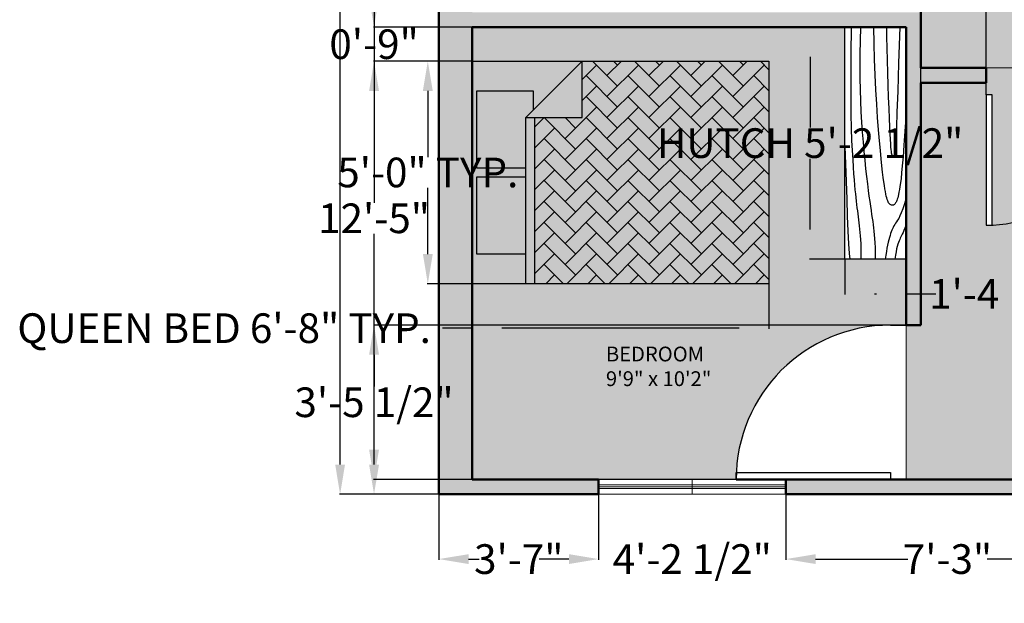
# Model space of a CAD drawing. Units: inches. Extents: x 339 to 824, y 73 to 445.
# Tile 1 of 5: x 339 to 605, y 73 to 230. Entities that reach past the tile are written whole.
import ezdxf

# ---------------------------------------------------------------- set-up
doc = ezdxf.new("R2010")
doc.units = ezdxf.units.IN
doc.header["$MEASUREMENT"] = 0
for name, color, linetype, lineweight in [('A-ANNO-DIMS', 2, 'Continuous', 18), ('A-AREA-IDEN', 7, 'Continuous', 25), ('A-DOOR', 3, 'Continuous', 25), ('A-FLOR-BNDY', 8, 'Continuous', 13), ('A-FLOR-PATT', 8, 'Continuous', 13), ('A-FURN', 9, 'Continuous', 25), ('A-FURN-FABR-PATT', 7, 'Continuous', 13), ('A-GLAZ', 4, 'Continuous', 18), ('A-WALL', 7, 'Continuous', 50), ('A-WALL-PATT', 1, 'Continuous', 13)]:
    doc.layers.add(name, color=color, linetype=linetype, lineweight=lineweight)
doc.layers.add('A-FURN-PATT', color=251, linetype='Continuous', lineweight=13, true_color=0x6d5f6c)
doc.styles.get("Standard").update_dxf_attribs({"font": 'arial.ttf'})
doc.dimstyles.get("Standard").update_dxf_attribs({"dimtxt": 8, "dimasz": 8, "dimexe": 0.18, "dimexo": 0.0625, "dimgap": 0.09, "dimtad": 0, "dimtih": 1, "dimtoh": 1, "dimdec": 0, "dimzin": 0, "dimdsep": 46, "dimlunit": 3, "dimtxsty": 'Standard', "dimcen": 0.09, "dimadec": 0, "dimazin": 0, "dimtfac": 1, "dimtdec": 0, "dimtofl": 0, "dimtmove": 0, "dimatfit": 3, "dimfxl": 1, "dimtolj": 1, "dimtzin": 0, "dimarcsym": 0})

# ---------------------------------------------------------------- blocks, each defined once
blk = doc.blocks.new('*U2')
for p, q in [((0, 0), (0, -6)), ((40, 0), (40, -6))]:
    blk.add_line(p, q)
blk.add_lwpolyline([(0, 0), (0, 40), (1.75, 40), (1.75, 0)], close=True)
blk.add_arc((0, 0), 40, 0, 90)
blk = doc.blocks.new('*U3')
for p, q in [((0, 0), (0, 6)), ((40, 0), (40, 6))]:
    blk.add_line(p, q)
blk.add_lwpolyline([(0, 0), (0, -40), (1.75, -40), (1.75, 0)], close=True)
blk.add_arc((0, 0), 40, 270, 0)
blk = doc.blocks.new('Hutch - 19 x 72 in.')
for p, q in [((0, -19), (0, 0)), ((0, 0), (71.999994, 0)), ((71.999994, 0), (71.999994, -19)), ((71.999994, -19), (0, -19))]:
    blk.add_line(p, q)
for points in [[(26.99999, 0), (32.30411, -0.35238), (36.66731, -0.66276), (40.20336, -0.93603), (43.02603, -1.17708), (45.2491, -1.39079), (46.98632, -1.58203), (48.35147, -1.7557), (49.45833, -1.91667), (50.40388, -2.06917), (51.21809, -2.21484), (51.91414, -2.35465), (52.5052, -2.48958), (53.00447, -2.6206), (53.42512, -2.7487), (53.78035, -2.87484), (54.08333, -3), (54.34537, -3.12516), (54.57031, -3.2513), (54.76008, -3.37939), (54.91666, -3.51042), (55.04198, -3.64534), (55.13801, -3.78516), (55.2067, -3.93083), (55.24999, -4.08333), (55.26904, -4.24316), (55.26171, -4.40885), (55.22509, -4.57845), (55.15624, -4.75), (55.05224, -4.92155), (54.91015, -5.09115), (54.72704, -5.25684), (54.49999, -5.41667), (54.22493, -5.56934), (53.89322, -5.71615), (53.49511, -5.85905), (53.02083, -6), (52.4606, -6.14095), (51.80468, -6.28385), (51.04329, -6.43066), (50.16666, -6.58333), (49.16007, -6.74381), (47.98892, -6.91406), (46.61368, -7.09603), (44.99478, -7.29167), (43.09268, -7.50293), (40.86783, -7.73177), (38.28067, -7.98014), (35.29166, -8.25), (31.87654, -8.54053), (28.07226, -8.83984), (23.93107, -9.1333), (19.5052, -9.40625), (14.84692, -9.64404), (10.00846, -9.83203), (5.04207, -9.95557), (0, -10)], [(52.99999, 0), (54.87133, -0.53955), (56.39257, -1.03516), (57.61205, -1.48975), (58.57812, -1.90625), (59.3391, -2.2876), (59.94335, -2.63672), (60.4392, -2.95654), (60.87499, -3.25), (61.29247, -3.52002), (61.70702, -3.76953), (62.12743, -4.00146), (62.56249, -4.21875), (63.02099, -4.42432), (63.51171, -4.62109), (64.04345, -4.81201), (64.62499, -5), (65.26489, -5.1875), (65.9707, -5.375), (66.74975, -5.5625), (67.60937, -5.75), (68.55688, -5.9375), (69.5996, -6.125), (70.744867, -6.3125), (71.999994, -6.5)], [(61.49999, 0), (62.35961, -0.35254), (63.08007, -0.66406), (63.68627, -0.94043), (64.20312, -1.1875), (64.65551, -1.41113), (65.06835, -1.61719), (65.46655, -1.81152), (65.87499, -2), (66.31762, -2.1875), (66.81445, -2.375), (67.38452, -2.5625), (68.04687, -2.75), (68.82055, -2.9375), (69.7246, -3.125), (70.77807, -3.3125), (71.999994, -3.5)], [(0, -2), (11.2006, -2.34123), (19.90169, -2.62044), (26.43969, -2.84595), (31.15103, -3.02604), (34.37214, -3.16903), (36.43945, -3.2832), (37.68936, -3.37687), (38.45833, -3.45833), (39.02937, -3.53459), (39.472, -3.60742), (39.80232, -3.67733), (40.03645, -3.74479), (40.1905, -3.8103), (40.28059, -3.87435), (40.32283, -3.93742), (40.33333, -4), (40.32405, -4.0625), (40.29036, -4.125), (40.22346, -4.1875), (40.11458, -4.25), (39.95491, -4.3125), (39.73567, -4.375), (39.44807, -4.4375), (39.08333, -4.5), (38.62491, -4.56282), (38.02538, -4.6276), (37.22957, -4.69629), (36.18228, -4.77083), (34.82836, -4.85319), (33.11262, -4.94531), (30.97989, -5.04915), (28.37499, -5.16667), (25.27416, -5.29818), (21.77929, -5.4375), (18.02368, -5.57682), (14.14062, -5.70833), (10.26342, -5.82422), (6.52539, -5.91667), (3.05981, -5.97786), (0, -6)], [(71.999994, -9.5), (70.071934, -9.51147), (68.38801, -9.54492), (66.91113, -9.59888), (65.60416, -9.67187), (64.43001, -9.76245), (63.35156, -9.86914), (62.3317, -9.99048), (61.33333, -10.125), (60.32128, -10.27157), (59.26822, -10.43034), (58.14876, -10.60181), (56.93749, -10.78646), (55.60904, -10.98478), (54.13801, -11.19726), (52.49902, -11.4244), (50.66666, -11.66667), (48.62239, -11.92358), (46.37499, -12.19075), (43.9401, -12.46281), (41.33333, -12.73437), (38.57031, -13.00008), (35.66666, -13.25456), (32.63801, -13.49243), (29.49999, -13.70833), (26.26367, -13.89689), (22.92187, -14.05273), (19.46289, -14.17049), (15.875, -14.24479), (12.14648, -14.27026), (8.26562, -14.24154), (4.2207, -14.15324), (0, -14)], [(0, -17), (8.37556, -17.14274), (15.58268, -17.20443), (21.74194, -17.19775), (26.97395, -17.13542), (31.39933, -17.03011), (35.13866, -16.89453), (38.31257, -16.74137), (41.04166, -16.58333), (43.4322, -16.43083), (45.5332, -16.28516), (47.37931, -16.14534), (49.0052, -16.01042), (50.44555, -15.87939), (51.73502, -15.7513), (52.90828, -15.62516), (53.99999, -15.5), (55.04044, -15.37508), (56.04231, -15.25065), (57.01391, -15.1272), (57.96353, -15.00521), (58.89949, -14.88517), (59.83007, -14.76758), (60.76358, -14.65291), (61.70833, -14.54167), (62.6752, -14.43465), (63.68554, -14.33398), (64.76326, -14.24211), (65.93229, -14.16146), (67.21655, -14.09448), (68.63997, -14.04362), (70.226475, -14.01131), (71.999994, -14)], [(36.99999, -19), (42.40038, -18.8125), (47.95312, -18.625), (53.43554, -18.4375), (58.62499, -18.25), (63.29882, -18.0625), (67.23437, -17.875), (70.208978, -17.6875), (71.999994, -17.5)]]:
    blk.add_lwpolyline(points)
blk = doc.blocks.new('Bed - Queen')
for p, q in [((0, -80.00003), (0, 0)), ((0, 0), (59.99999, 0)), ((59.99999, 0), (59.99999, -80.00003)), ((7.99999, -1.2), (28.79998, -1.2)), ((7.99999, -14.4), (7.99999, -1.2)), ((28.79998, -1.2), (28.79998, -14.4)), ((31.19999, -1.2), (51.99999, -1.2)), ((31.19999, -14.4), (31.19999, -1.2)), ((51.99999, -1.2), (51.99999, -16.4)), ((0, -14.4), (44.8, -14.4)), ((59.99999, -29.6), (44.8, -14.4)), ((44.8, -14.4), (44.8, -29.6)), ((44.8, -16.8), (0, -16.8)), ((51.99999, -16.4), (46.79936, -16.4)), ((44.8, -29.6), (59.99999, -29.6)), ((59.99999, -80.00003), (0, -80.00003))]:
    blk.add_line(p, q)
blk = doc.blocks.new('*D12')
at = {"layer": 'A-ANNO-DIMS', "color": 0, "lineweight": -2, "transparency": 16777216}
for p, q in [((452.42, 416.06), (425.65, 416.06)), ((425.83, 408.06), (425.83, 263.23)), ((425.83, 110.06), (425.83, 254.89)), ((452.42, 102.06), (425.65, 102.06))]:
    blk.add_line(p, q, dxfattribs=at)
at = {"layer": 'A-ANNO-DIMS', "color": 0, "transparency": 16777216}
for points in [[(424.5, 408.06), (427.16, 408.06), (425.83, 416.06)], [(424.5, 110.06), (427.16, 110.06), (425.83, 102.06)]]:
    blk.add_solid(points, dxfattribs=at)
at = {"layer": 'Defpoints', "color": 0, "transparency": 16777216}
for p in [(452.48, 416.06), (425.83, 102.06), (452.48, 102.06)]:
    blk.add_point(p, dxfattribs=at)
at = {"layer": 'A-ANNO-DIMS', "color": 0, "transparency": 16777216, "insert": (425.83, 259.06), "char_height": 8, "attachment_point": 5}
blk.add_mtext('\\A1;26\'-2"', dxfattribs=at)
blk = doc.blocks.new('*D14')
at = {"layer": 'A-ANNO-DIMS', "color": 0, "lineweight": -2, "transparency": 16777216}
for p, q in [((461.48, 158.79), (461.48, 146.67)), ((541.48, 158.79), (541.48, 146.67)), ((461.48, 146.85), (453.48, 146.85)), ((533.48, 146.85), (469.48, 146.85))]:
    blk.add_line(p, q, dxfattribs=at)
at = {"layer": 'A-ANNO-DIMS', "color": 0, "transparency": 16777216}
for points in [[(469.48, 148.18), (469.48, 145.51), (461.48, 146.85)], [(533.48, 148.18), (533.48, 145.51), (541.48, 146.85)]]:
    blk.add_solid(points, dxfattribs=at)
at = {"layer": 'Defpoints', "color": 0, "transparency": 16777216}
for p in [(461.48, 158.85), (541.48, 158.85), (461.48, 146.85)]:
    blk.add_point(p, dxfattribs=at)
at = {"layer": 'A-ANNO-DIMS', "color": 0, "transparency": 16777216, "insert": (394.55, 146.85), "char_height": 8, "attachment_point": 5}
blk.add_mtext('\\A1;QUEEN BED 6\'-8" TYP.', dxfattribs=at)
blk = doc.blocks.new('*D15')
at = {"layer": 'A-ANNO-DIMS', "color": 0, "lineweight": -2, "transparency": 16777216}
for p, q in [((461.42, 218.85), (449.3, 218.85)), ((449.48, 210.85), (449.48, 193.02)), ((449.48, 166.85), (449.48, 184.67)), ((461.42, 158.85), (449.3, 158.85))]:
    blk.add_line(p, q, dxfattribs=at)
at = {"layer": 'A-ANNO-DIMS', "color": 0, "transparency": 16777216}
for points in [[(448.15, 210.85), (450.82, 210.85), (449.48, 218.85)], [(448.15, 166.85), (450.82, 166.85), (449.48, 158.85)]]:
    blk.add_solid(points, dxfattribs=at)
at = {"layer": 'Defpoints', "color": 0, "transparency": 16777216}
for p in [(449.48, 218.85), (461.48, 218.85), (461.48, 158.85)]:
    blk.add_point(p, dxfattribs=at)
at = {"layer": 'A-ANNO-DIMS', "color": 0, "transparency": 16777216, "insert": (449.48, 188.85), "char_height": 8, "attachment_point": 5}
blk.add_mtext('\\A1;5\'-0" TYP.', dxfattribs=at)
blk = doc.blocks.new('*D16')
at = {"layer": 'A-ANNO-DIMS', "color": 0, "lineweight": -2, "transparency": 16777216}
for p, q in [((561.9, 228.06), (552.4, 228.06)), ((552.58, 220.06), (552.58, 200.99)), ((552.58, 173.46), (552.58, 192.54)), ((561.9, 165.46), (552.4, 165.46))]:
    blk.add_line(p, q, dxfattribs=at)
at = {"layer": 'A-ANNO-DIMS', "color": 0, "transparency": 16777216}
for points in [[(551.24, 220.06), (553.91, 220.06), (552.58, 228.06)], [(551.24, 173.46), (553.91, 173.46), (552.58, 165.46)]]:
    blk.add_solid(points, dxfattribs=at)
at = {"layer": 'Defpoints', "color": 0, "transparency": 16777216}
for p in [(561.97, 228.06), (552.58, 165.46), (561.97, 165.46)]:
    blk.add_point(p, dxfattribs=at)
at = {"layer": 'A-ANNO-DIMS', "color": 0, "transparency": 16777216, "insert": (552.58, 196.76), "char_height": 8, "attachment_point": 5}
blk.add_mtext('\\A1;HUTCH 5\'-2 1/2"', dxfattribs=at)
blk = doc.blocks.new('*D17')
at = {"layer": 'A-ANNO-DIMS', "color": 0, "lineweight": -2, "transparency": 16777216}
for p, q in [((561.97, 165.4), (561.97, 155.9)), ((578.48, 165.4), (578.48, 155.9)), ((569.97, 156.08), (570.48, 156.08)), ((578.48, 156.08), (586.48, 156.08))]:
    blk.add_line(p, q, dxfattribs=at)
at = {"layer": 'A-ANNO-DIMS', "color": 0, "transparency": 16777216}
for points in [[(569.97, 157.41), (569.97, 154.74), (561.97, 156.08)], [(570.48, 157.41), (570.48, 154.74), (578.48, 156.08)]]:
    blk.add_solid(points, dxfattribs=at)
at = {"layer": 'Defpoints', "color": 0, "transparency": 16777216}
for p in [(561.97, 165.46), (578.48, 165.46), (578.48, 156.08)]:
    blk.add_point(p, dxfattribs=at)
at = {"layer": 'A-ANNO-DIMS', "color": 0, "transparency": 16777216, "insert": (606.15, 156.08), "char_height": 8, "attachment_point": 5}
blk.add_mtext('\\A1;1\'-4 1/2"', dxfattribs=at)
blk = doc.blocks.new('*D30')
at = {"layer": 'A-ANNO-DIMS', "color": 0, "lineweight": -2, "transparency": 16777216}
for p, q in [((452.48, 102), (452.48, 84.38)), ((495.53, 102), (495.53, 84.38)), ((460.48, 84.56), (463.29, 84.56)), ((487.53, 84.56), (484.73, 84.56))]:
    blk.add_line(p, q, dxfattribs=at)
at = {"layer": 'A-ANNO-DIMS', "color": 0, "transparency": 16777216}
for points in [[(460.48, 85.89), (460.48, 83.23), (452.48, 84.56)], [(487.53, 85.89), (487.53, 83.23), (495.53, 84.56)]]:
    blk.add_solid(points, dxfattribs=at)
at = {"layer": 'Defpoints', "color": 0, "transparency": 16777216}
for p in [(452.48, 102.06), (495.53, 102.06), (495.53, 84.56)]:
    blk.add_point(p, dxfattribs=at)
at = {"layer": 'A-ANNO-DIMS', "color": 0, "transparency": 16777216, "insert": (474.01, 84.56), "char_height": 8, "attachment_point": 5}
blk.add_mtext('\\A1;3\'-7"', dxfattribs=at)
blk = doc.blocks.new('*D31')
at = {"layer": 'A-ANNO-DIMS', "color": 0, "lineweight": -2, "transparency": 16777216}
for p, q in [((495.53, 102), (495.53, 84.38)), ((546.07, 102), (546.07, 84.38)), ((487.53, 84.56), (479.53, 84.56)), ((554.07, 84.56), (562.07, 84.56))]:
    blk.add_line(p, q, dxfattribs=at)
at = {"layer": 'A-ANNO-DIMS', "color": 0, "transparency": 16777216}
for points in [[(487.53, 85.89), (487.53, 83.23), (495.53, 84.56)], [(554.07, 85.89), (554.07, 83.23), (546.07, 84.56)]]:
    blk.add_solid(points, dxfattribs=at)
at = {"layer": 'Defpoints', "color": 0, "transparency": 16777216}
for p in [(495.53, 102.06), (546.07, 102.06), (546.07, 84.56)]:
    blk.add_point(p, dxfattribs=at)
at = {"layer": 'A-ANNO-DIMS', "color": 0, "transparency": 16777216, "insert": (520.8, 84.56), "char_height": 8, "attachment_point": 5}
blk.add_mtext('\\A1;4\'-2 1/2"', dxfattribs=at)
blk = doc.blocks.new('*D32')
at = {"layer": 'A-ANNO-DIMS', "color": 0, "lineweight": -2, "transparency": 16777216}
for p, q in [((546.07, 102), (546.07, 84.38)), ((633.18, 102), (633.18, 84.38)), ((554.07, 84.56), (578.93, 84.56)), ((625.18, 84.56), (600.31, 84.56))]:
    blk.add_line(p, q, dxfattribs=at)
at = {"layer": 'A-ANNO-DIMS', "color": 0, "transparency": 16777216}
for points in [[(554.07, 85.89), (554.07, 83.23), (546.07, 84.56)], [(625.18, 85.89), (625.18, 83.23), (633.18, 84.56)]]:
    blk.add_solid(points, dxfattribs=at)
at = {"layer": 'Defpoints', "color": 0, "transparency": 16777216}
for p in [(546.07, 102.06), (633.18, 102.06), (633.18, 84.56)]:
    blk.add_point(p, dxfattribs=at)
at = {"layer": 'A-ANNO-DIMS', "color": 0, "transparency": 16777216, "insert": (589.62, 84.56), "char_height": 8, "attachment_point": 5}
blk.add_mtext('\\A1;7\'-3"', dxfattribs=at)
blk = doc.blocks.new('*D34')
at = {"layer": 'A-ANNO-DIMS', "color": 0, "lineweight": -2, "transparency": 16777216}
for p, q in [((452.42, 250.91), (434.8, 250.91)), ((434.98, 242.91), (434.98, 180.66)), ((434.98, 110.06), (434.98, 172.31)), ((452.42, 102.06), (434.8, 102.06))]:
    blk.add_line(p, q, dxfattribs=at)
at = {"layer": 'A-ANNO-DIMS', "color": 0, "transparency": 16777216}
for points in [[(433.65, 242.91), (436.32, 242.91), (434.98, 250.91)], [(433.65, 110.06), (436.32, 110.06), (434.98, 102.06)]]:
    blk.add_solid(points, dxfattribs=at)
at = {"layer": 'Defpoints', "color": 0, "transparency": 16777216}
for p in [(434.98, 250.91), (452.48, 250.91), (452.48, 102.06)]:
    blk.add_point(p, dxfattribs=at)
at = {"layer": 'A-ANNO-DIMS', "color": 0, "transparency": 16777216, "insert": (434.98, 176.48), "char_height": 8, "attachment_point": 5}
blk.add_mtext('\\A1;12\'-5"', dxfattribs=at)
blk = doc.blocks.new('*D38')
at = {"layer": 'A-ANNO-DIMS', "color": 0, "lineweight": -2, "transparency": 16777216}
for p, q in [((592.11, 433.56), (584.11, 433.56)), ((600.11, 213.12), (600.11, 433.74)), ((635.29, 213.12), (635.29, 433.74)), ((643.29, 433.56), (651.29, 433.56))]:
    blk.add_line(p, q, dxfattribs=at)
at = {"layer": 'A-ANNO-DIMS', "color": 0, "transparency": 16777216}
for points in [[(592.11, 434.89), (592.11, 432.23), (600.11, 433.56)], [(643.29, 434.89), (643.29, 432.23), (635.29, 433.56)]]:
    blk.add_solid(points, dxfattribs=at)
at = {"layer": 'Defpoints', "color": 0, "transparency": 16777216}
for p in [(635.29, 433.56), (600.11, 213.06), (635.29, 213.06)]:
    blk.add_point(p, dxfattribs=at)
at = {"layer": 'A-ANNO-DIMS', "color": 0, "transparency": 16777216, "insert": (617.7, 433.56), "char_height": 8, "attachment_point": 5}
blk.add_mtext('\\A1;2\'-11"', dxfattribs=at)
blk = doc.blocks.new('*D40')
at = {"layer": 'A-ANNO-DIMS', "color": 0, "lineweight": -2, "transparency": 16777216}
for p, q in [((578.42, 147.67), (434.8, 147.67)), ((434.98, 139.67), (434.98, 131.09)), ((434.98, 114.06), (434.98, 122.63)), ((578.42, 106.06), (434.8, 106.06))]:
    blk.add_line(p, q, dxfattribs=at)
at = {"layer": 'A-ANNO-DIMS', "color": 0, "transparency": 16777216}
for points in [[(433.65, 139.67), (436.32, 139.67), (434.98, 147.67)], [(433.65, 114.06), (436.32, 114.06), (434.98, 106.06)]]:
    blk.add_solid(points, dxfattribs=at)
at = {"layer": 'Defpoints', "color": 0, "transparency": 16777216}
for p in [(578.48, 147.67), (434.98, 106.06), (578.48, 106.06)]:
    blk.add_point(p, dxfattribs=at)
at = {"layer": 'A-ANNO-DIMS', "color": 0, "transparency": 16777216, "insert": (434.98, 126.86), "char_height": 8, "attachment_point": 5}
blk.add_mtext('\\A1;3\'-5 1/2"', dxfattribs=at)
blk = doc.blocks.new('*D55')
at = {"layer": 'A-ANNO-DIMS', "color": 0, "lineweight": -2, "transparency": 16777216}
for p, q in [((582.48, 213.12), (582.48, 433.74)), ((590.48, 433.56), (592.11, 433.56)), ((600.11, 213.12), (600.11, 433.74)), ((600.11, 433.56), (608.11, 433.56))]:
    blk.add_line(p, q, dxfattribs=at)
at = {"layer": 'A-ANNO-DIMS', "color": 0, "transparency": 16777216}
for points in [[(590.48, 434.89), (590.48, 432.23), (582.48, 433.56)], [(592.11, 434.89), (592.11, 432.23), (600.11, 433.56)]]:
    blk.add_solid(points, dxfattribs=at)
at = {"layer": 'Defpoints', "color": 0, "transparency": 16777216}
for p in [(600.11, 433.56), (582.48, 213.06), (600.11, 213.06)]:
    blk.add_point(p, dxfattribs=at)
at = {"layer": 'A-ANNO-DIMS', "color": 0, "transparency": 16777216, "insert": (627.78, 433.56), "char_height": 8, "attachment_point": 5}
blk.add_mtext('\\A1;1\'-5 1/2"', dxfattribs=at)
blk = doc.blocks.new('*D62')
at = {"layer": 'A-ANNO-DIMS', "color": 0, "lineweight": -2, "transparency": 16777216}
for p, q in [((434.98, 236.06), (434.98, 244.06)), ((461.42, 228.06), (434.8, 228.06)), ((461.42, 218.85), (434.8, 218.85)), ((434.98, 210.85), (434.98, 202.85))]:
    blk.add_line(p, q, dxfattribs=at)
at = {"layer": 'A-ANNO-DIMS', "color": 0, "transparency": 16777216}
for points in [[(433.65, 236.06), (436.32, 236.06), (434.98, 228.06)], [(433.65, 210.85), (436.32, 210.85), (434.98, 218.85)]]:
    blk.add_solid(points, dxfattribs=at)
at = {"layer": 'Defpoints', "color": 0, "transparency": 16777216}
for p in [(461.48, 228.06), (434.98, 218.85), (461.48, 218.85)]:
    blk.add_point(p, dxfattribs=at)
at = {"layer": 'A-ANNO-DIMS', "color": 0, "transparency": 16777216, "insert": (434.98, 223.45), "char_height": 8, "attachment_point": 5}
blk.add_mtext('\\A1;0\'-9"', dxfattribs=at)

msp = doc.modelspace()

# ---------------------------------------------------------------- hatches: boundary and pattern name
at = {"layer": 'A-FLOR-PATT'}
h = msp.add_hatch(color=256, dxfattribs=at)
h.dxf.hatch_style = 1
h.paths.add_polyline_path([(661.42, 241.56), (665.51, 241.56, -0.414214), (667.55, 243.6), (678.83, 243.6, -0.414214), (680.87, 241.56, -0.414214), (682.91, 243.6), (696.76, 243.6, -0.414214), (698.8, 241.56, -0.414214), (700.84, 243.6), (714.97, 243.6, -0.412935), (717.02, 241.56, -0.410727), (719.02, 243.61, -0.419077), (716.95, 245.66), (716.95, 259.06, -0.414214), (718.99, 261.11, -0.414214), (716.95, 263.15), (716.95, 274.6, -0.414214), (718.99, 276.64), (718.99, 280.73, -0.414214), (720.01, 281.75), (743.48, 281.75), (743.48, 293.36), (743.48, 299.72), (741.87, 299.72), (741.87, 299.75, -0.401453), (706.66, 336.54), (706.66, 342.06), (582.48, 342.06), (582.48, 307.06), (582.48, 217.06), (635.29, 217.06), (660.4, 217.06), (660.4, 240.53, -0.414214)])
h.paths.add_polyline_path([(639.94, 279.04), (679.09, 279.04), (679.09, 293.92), (639.94, 293.92)], flags=24)
h = msp.add_hatch(color=256, dxfattribs=at)
h.dxf.hatch_style = 1
h.paths.add_polyline_path([(495.53, 106.06), (532.64, 106.06), (532.64, 107.88), (532.68, 107.88, -0.401453), (574.24, 147.66), (578.48, 147.66), (578.48, 147.67), (578.48, 165.46), (561.97, 165.46), (561.97, 228.06), (461.48, 228.06), (461.48, 218.85), (541.48, 218.85), (541.48, 158.85), (461.48, 158.85), (461.48, 106.06)])
h.paths.add_polyline_path([(496.11, 128.97), (526.9, 128.97), (526.9, 143.86), (496.11, 143.86)], flags=24)
h = msp.add_hatch(color=256, dxfattribs=at)
h.dxf.hatch_style = 1
h.paths.add_polyline_path([(578.48, 106.06), (710.48, 106.06), (710.48, 130.47), (706.48, 130.47), (706.48, 137.8), (692.06, 137.8), (692.06, 195.19), (670.62, 195.11), (670.62, 213.06), (635.29, 213.06), (635.29, 217.06), (600.11, 217.06), (600.11, 213.06), (582.48, 213.06), (582.48, 147.67), (578.48, 147.67)])
h.paths.add_polyline_path([(600.11, 174.62), (600.11, 209.78), (601.65, 209.78), (601.65, 174.62)], flags=16)
h.paths.add_polyline_path([(630.19, 155.1), (658.99, 155.1), (658.99, 168.27), (630.19, 168.27)], flags=24)
h = msp.add_hatch(color=256, dxfattribs=at)
h.dxf.hatch_style = 1
h.paths.add_polyline_path([(710.48, 106.06), (710.48, 130.47), (706.48, 130.47), (706.48, 137.8), (692.06, 137.8), (692.06, 195.19), (670.62, 195.11), (670.62, 213.06), (635.29, 213.06), (635.29, 217.06), (600.11, 217.06), (600.11, 213.06), (582.48, 213.06), (582.48, 147.67), (582.91, 106.06)])
h.paths.add_polyline_path([(601.65, 174.62), (600.11, 174.62), (600.11, 209.78), (601.65, 209.78)], flags=16)
h.paths.add_polyline_path([(630.19, 155.1), (658.99, 155.1), (658.99, 168.27), (630.19, 168.27)], flags=24)
at = {"layer": 'A-FURN-FABR-PATT'}
h = msp.add_hatch(dxfattribs=at)
h.set_pattern_fill('AR-HBONE', color=256)
h.paths.add_polyline_path([(478.28, 158.85), (541.48, 158.85), (541.48, 218.85), (491.08, 218.85), (491.08, 203.65), (478.28, 203.65)])
at = {"layer": 'A-FURN-PATT'}
h = msp.add_hatch(color=256, dxfattribs=at)
h.dxf.hatch_style = 1
h.paths.add_polyline_path([(491.08, 218.85), (461.48, 218.85), (461.48, 158.85), (475.88, 158.85), (475.88, 166.85), (462.68, 166.85), (462.68, 187.65), (475.88, 187.65), (475.88, 190.05), (462.68, 190.05), (462.68, 210.85), (477.88, 210.85), (477.88, 205.65)])
h = msp.add_hatch(color=256, dxfattribs=at)
h.dxf.hatch_style = 1
h.paths.add_polyline_path([(475.88, 203.65), (491.08, 203.65), (491.08, 218.85)])
h = msp.add_hatch(color=256, dxfattribs=at)
h.dxf.hatch_style = 1
h.paths.add_polyline_path([(491.08, 218.85), (491.08, 203.65), (478.28, 203.65), (478.28, 158.85), (541.48, 158.85), (541.48, 218.85)])
h = msp.add_hatch(color=256, dxfattribs=at)
h.dxf.hatch_style = 1
h.paths.add_polyline_path([(475.88, 203.65), (477.88, 205.65), (477.88, 210.85), (462.68, 210.85), (462.68, 190.05), (475.88, 190.05)])
h = msp.add_hatch(color=256, dxfattribs=at)
h.dxf.hatch_style = 1
h.paths.add_polyline_path([(478.28, 203.65), (475.88, 203.65), (475.88, 158.85), (478.28, 158.85)])
h = msp.add_hatch(color=256, dxfattribs=at)
h.dxf.hatch_style = 1
h.paths.add_polyline_path([(475.88, 187.65), (462.68, 187.65), (462.68, 166.85), (475.88, 166.85)])
at = {"layer": 'A-WALL-PATT'}
h = msp.add_hatch(color=256, dxfattribs=at)
h.dxf.hatch_style = 1
h.paths.add_polyline_path([(452.48, 102.06), (495.53, 102.06), (495.53, 106.06), (461.48, 106.06), (461.48, 228.06), (578.48, 228.06), (578.48, 165.46), (578.48, 147.67), (582.48, 147.67), (582.48, 213.06), (600.11, 213.06), (600.11, 215.06), (600.11, 217.06), (582.48, 217.06), (582.48, 232.06), (461.48, 232.06), (461.48, 250.91), (452.48, 250.91)])
h = msp.add_hatch(color=256, dxfattribs=at)
h.dxf.hatch_style = 1
h.paths.add_polyline_path([(546.07, 106.06), (546.07, 102.06), (633.18, 102.06), (633.18, 106.06), (625.18, 106.06)])

# ---------------------------------------------------------------- linework, layer by layer
at = {"layer": 'A-FLOR-BNDY'}
for p, q in [((582.48, 217.06), (635.29, 217.06)), ((578.48, 181.98), (578.48, 106.06))]:
    msp.add_line(p, q, dxfattribs=at)
at = {"layer": 'A-GLAZ'}
for p, q in [((495.53, 106.06), (546.07, 106.06)), ((495.53, 104.56), (546.07, 104.56)), ((495.53, 104.06), (546.07, 104.06)), ((520.8, 106.06), (520.8, 102.06)), ((495.53, 103.56), (546.07, 103.56)), ((495.53, 102.06), (546.07, 102.06))]:
    msp.add_line(p, q, dxfattribs=at)
at = {"layer": 'A-WALL'}
for p, q in [((582.48, 217.06), (582.48, 307.06)), ((452.48, 102.06), (452.48, 250.91)), ((461.48, 106.06), (461.48, 228.06)), ((461.48, 228.06), (578.48, 228.06)), ((578.48, 147.67), (578.48, 228.06)), ((582.48, 217.06), (600.11, 217.06)), ((600.11, 213.06), (600.11, 217.06)), ((582.48, 147.67), (582.48, 213.06)), ((582.48, 213.06), (600.11, 213.06)), ((578.48, 147.67), (582.48, 147.67)), ((461.48, 106.06), (495.53, 106.06)), ((495.53, 106.06), (495.53, 102.06)), ((532.64, 106.06), (633.18, 106.06)), ((546.07, 106.06), (546.07, 102.06)), ((546.07, 106.06), (578.48, 106.06)), ((578.48, 106.06), (743.48, 106.06)), ((452.48, 102.06), (495.53, 102.06)), ((546.07, 102.06), (633.18, 102.06))]:
    msp.add_line(p, q, dxfattribs=at)

# ---------------------------------------------------------------- block references
at = {"layer": 'A-DOOR', "xscale": 0.8792070118950395, "yscale": 0.8792070118950395, "zscale": 0.8792070118950395}
msp.add_blockref('*U3', (600.11, 209.78), dxfattribs=at)
at = {"layer": 'A-DOOR', "xscale": 1.040017593541602, "yscale": 1.040017593541602, "zscale": 1.040017593541602, "rotation": 90}
msp.add_blockref('*U2', (574.24, 106.06), dxfattribs=at)
at = {"layer": 'A-FURN', "xscale": 0.869379546477353, "yscale": 0.869379546477353, "zscale": 0.869379546477353, "rotation": 270}
msp.add_blockref('Hutch - 19 x 72 in.', (578.48, 228.06), dxfattribs=at)
at = {"layer": 'A-FURN', "rotation": 90}
msp.add_blockref('Bed - Queen', (461.48, 158.85), dxfattribs=at)

# ---------------------------------------------------------------- texts
at = {"layer": 'A-AREA-IDEN', "insert": (497.52, 141.87), "char_height": 3.9887, "attachment_point": 1}
msp.add_mtext_dynamic_manual_height_columns('BEDROOM \\P9\'9" x 10\'2"', width=44.4226, gutter_width=19.94, heights=[0], dxfattribs=at)

# ---------------------------------------------------------------- dimensions: what is measured, and where the dimension line sits
at = {"layer": 'A-ANNO-DIMS'}
for base, p1, p2, picture, middle in [((600.11, 433.56), (582.48, 213.06), (600.11, 213.06), '*D55', (627.78, 433.56)), ((635.29, 433.56), (600.11, 213.06), (635.29, 213.06), '*D38', (617.7, 433.56)), ((578.48, 156.08), (561.97, 165.46), (578.48, 165.46), '*D17', (606.15, 156.08)), ((495.5324, 84.5602), (452.4839, 102.0602), (495.5324, 102.0602), '*D30', (474.0082, 84.5602)), ((546.07, 84.56), (495.53, 102.06), (546.07, 102.06), '*D31', (520.8, 84.56)), ((633.18, 84.56), (546.07, 102.06), (633.18, 102.06), '*D32', (589.62, 84.56))]:
    dim = msp.add_linear_dim(base=base, p1=p1, p2=p2, dimstyle='Standard', override={"dimdec": 1, "dimlfac": 1, "dimrnd": 0, "dimzin": 1, "dimdsep": 46, "dimlunit": 4, "dimfrac": 2}, dxfattribs=at)
    dim.commit()
    dim.dimension.update_dxf_attribs({"geometry": picture, "text_midpoint": middle})
for base, p1, p2, override, picture, middle in [((425.83, 102.06), (452.48, 416.06), (452.48, 102.06), {"dimclrd": 0, "dimclre": 0, "dimclrt": 0}, '*D12', (425.83, 259.06)), ((434.9839, 250.9061), (452.4839, 102.0602), (452.4839, 250.9061), {"dimdec": 1, "dimlfac": 1, "dimrnd": 0, "dimzin": 1, "dimdsep": 46, "dimlunit": 4, "dimfrac": 2}, '*D34', (434.9839, 176.4832)), ((434.98, 218.85), (461.48, 228.06), (461.48, 218.85), {"dimdec": 1, "dimlfac": 1, "dimrnd": 0, "dimzin": 1, "dimdsep": 46, "dimlunit": 4, "dimfrac": 2}, '*D62', (434.98, 223.45)), ((434.98, 106.06), (578.48, 147.67), (578.48, 106.06), {"dimdec": 1, "dimlfac": 1, "dimrnd": 0, "dimzin": 1, "dimdsep": 46, "dimlunit": 4, "dimfrac": 2}, '*D40', (434.98, 126.86))]:
    dim = msp.add_linear_dim(base=base, p1=p1, p2=p2, angle=90, dimstyle='Standard', override=override, dxfattribs=at)
    dim.commit()
    dim.dimension.update_dxf_attribs({"geometry": picture, "text_midpoint": middle})
for base, p1, p2, angle, text, picture, middle in [((552.58, 165.46), (561.97, 228.06), (561.97, 165.46), 270, 'HUTCH <>', '*D16', (552.58, 196.76)), ((449.48, 218.85), (461.48, 158.85), (461.48, 218.85), 90, '<> TYP.', '*D15', (449.48, 188.85)), ((461.48, 146.85), (541.48, 158.85), (461.48, 158.85), 180, 'QUEEN BED <> TYP.', '*D14', (394.55, 146.85))]:
    dim = msp.add_linear_dim(base=base, p1=p1, p2=p2, angle=angle, text=text, dimstyle='Standard', override={"dimdec": 1, "dimlfac": 1, "dimrnd": 0, "dimzin": 1, "dimdsep": 46, "dimlunit": 4, "dimfrac": 2}, dxfattribs=at)
    dim.commit()
    dim.dimension.update_dxf_attribs({"geometry": picture, "text_midpoint": middle})

doc.saveas('drawing.dxf')
